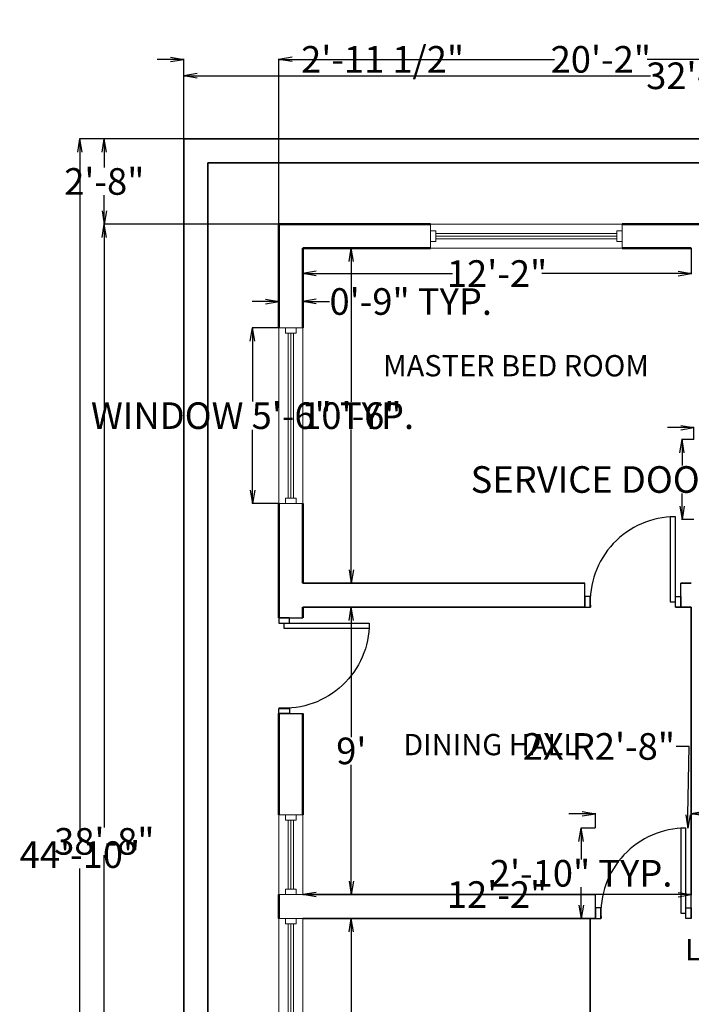
# Model space of a CAD drawing. Units: inches. Extents: x -6539 to -6057, y 19106 to 19733.
# Tile 2 of 3: x -6539 to -6286, y 19363 to 19733. Entities that reach past the tile are written whole.
import ezdxf

# ---------------------------------------------------------------- set-up
doc = ezdxf.new("R2010")
doc.units = ezdxf.units.IN
doc.header["$MEASUREMENT"] = 0
for name, color, linetype, lineweight in [('A-ANNO-DIMS', 121, 'Continuous', 18), ('A-AREA-IDEN', 250, 'Continuous', 25), ('A-WALL-EXTR', 222, 'Continuous', 50), ('C-PROP-WALL', 140, 'Continuous', 35), ('DOORS', 3, 'Continuous', 25), ('interior WALLS', 222, 'Continuous', 35), ('WINDOWS', 20, 'Continuous', 18)]:
    doc.layers.add(name, color=color, linetype=linetype, lineweight=lineweight)
doc.styles.get("Standard").update_dxf_attribs({"font": 'arial.ttf'})
doc.dimstyles.get("Standard").update_dxf_attribs({"dimtxt": 10, "dimasz": 5, "dimexe": 0.18, "dimexo": 0.0625, "dimgap": 0.09, "dimtad": 0, "dimtih": 1, "dimtoh": 1, "dimdec": 0, "dimzin": 0, "dimdsep": 46, "dimlunit": 4, "dimtxsty": 'Standard', "dimblk": 'OPEN', "dimcen": 0.09, "dimadec": 0, "dimazin": 0, "dimtfac": 1, "dimtdec": 0, "dimtofl": 0, "dimtmove": 0, "dimatfit": 0, "dimfxl": 1, "dimtolj": 1, "dimtzin": 0, "dimarcsym": 0})

# ---------------------------------------------------------------- blocks, each defined once
blk = doc.blocks.new('_Open')
at = {"color": 0, "linetype": 'ByBlock', "lineweight": -2}
for p, q in [((-1, 0.167), (0, 0)), ((-1, -0.167), (0, 0)), ((0, 0), (-1, 0))]:
    blk.add_line(p, q, dxfattribs=at)
blk = doc.blocks.new('*D2')
at = {"layer": 'A-ANNO-DIMS', "color": 0, "lineweight": -2, "transparency": 16777216}
for p, q in [((-6476.93, 19688.68), (-6476.93, 19712.48)), ((-6471.93, 19712.3), (-6301.58, 19712.3)), ((-6096.7, 19712.3), (-6267.05, 19712.3)), ((-6091.7, 19688.68), (-6091.7, 19712.48))]:
    blk.add_line(p, q, dxfattribs=at)
at = {"layer": 'Defpoints', "color": 0, "transparency": 16777216}
for p in [(-6091.7, 19712.3), (-6476.93, 19688.62), (-6091.7, 19688.62)]:
    blk.add_point(p, dxfattribs=at)
at = {"layer": 'A-ANNO-DIMS', "color": 0, "lineweight": -2, "transparency": 16777216, "xscale": 5, "yscale": 5, "zscale": 5, "rotation": 180}
blk.add_blockref('_Open', (-6476.93, 19712.3), dxfattribs=at)
at = {"layer": 'A-ANNO-DIMS', "color": 0, "lineweight": -2, "transparency": 16777216, "xscale": 5, "yscale": 5, "zscale": 5}
blk.add_blockref('_Open', (-6091.7, 19712.3), dxfattribs=at)
at = {"layer": 'A-ANNO-DIMS', "color": 0, "transparency": 16777216, "insert": (-6284.31, 19712.3), "char_height": 10, "attachment_point": 5}
blk.add_mtext('\\A1;32\'-1"', dxfattribs=at)
blk = doc.blocks.new('*D3')
at = {"layer": 'A-ANNO-DIMS', "color": 0, "lineweight": -2, "transparency": 16777216}
for p, q in [((-6476.99, 19688.62), (-6516.12, 19688.62)), ((-6515.94, 19683.62), (-6515.94, 19424.78)), ((-6515.94, 19155.56), (-6515.94, 19414.39)), ((-6476.99, 19150.56), (-6516.12, 19150.56))]:
    blk.add_line(p, q, dxfattribs=at)
at = {"layer": 'Defpoints', "color": 0, "transparency": 16777216}
for p in [(-6515.94, 19688.62), (-6476.93, 19688.62), (-6476.93, 19150.56)]:
    blk.add_point(p, dxfattribs=at)
at = {"layer": 'A-ANNO-DIMS', "color": 0, "lineweight": -2, "transparency": 16777216, "xscale": 5, "yscale": 5, "zscale": 5}
for p, rotation in [((-6515.94, 19688.62), 90), ((-6515.94, 19150.56), 270)]:
    blk.add_blockref('_Open', p, dxfattribs=dict(at, rotation=rotation))
at = {"layer": 'A-ANNO-DIMS', "color": 0, "transparency": 16777216, "insert": (-6515.94, 19419.59), "char_height": 10, "attachment_point": 5}
blk.add_mtext('\\A1;44\'-10"', dxfattribs=at)
blk = doc.blocks.new('*D6')
at = {"layer": 'A-ANNO-DIMS', "color": 0, "lineweight": -2, "transparency": 16777216}
for p, q in [((-6432.2, 19647.5), (-6432.2, 19637.79)), ((-6286.2, 19647.5), (-6286.2, 19637.79)), ((-6427.2, 19637.97), (-6376, 19637.97)), ((-6291.2, 19637.97), (-6342.41, 19637.97))]:
    blk.add_line(p, q, dxfattribs=at)
at = {"layer": 'Defpoints', "color": 0, "transparency": 16777216}
for p in [(-6432.2, 19647.56), (-6286.2, 19647.56), (-6286.2, 19637.97)]:
    blk.add_point(p, dxfattribs=at)
at = {"layer": 'A-ANNO-DIMS', "color": 0, "lineweight": -2, "transparency": 16777216, "xscale": 5, "yscale": 5, "zscale": 5, "rotation": 180}
blk.add_blockref('_Open', (-6432.2, 19637.97), dxfattribs=at)
at = {"layer": 'A-ANNO-DIMS', "color": 0, "lineweight": -2, "transparency": 16777216, "xscale": 5, "yscale": 5, "zscale": 5}
blk.add_blockref('_Open', (-6286.2, 19637.97), dxfattribs=at)
at = {"layer": 'A-ANNO-DIMS', "color": 0, "transparency": 16777216, "insert": (-6359.2, 19637.97), "char_height": 10, "attachment_point": 5}
blk.add_mtext('\\A1;12\'-2"', dxfattribs=at)
blk = doc.blocks.new('*D9')
at = {"layer": 'A-ANNO-DIMS', "color": 0, "lineweight": -2, "transparency": 16777216}
for p, q in [((-6432.14, 19647.56), (-6413.78, 19647.56)), ((-6413.96, 19642.56), (-6413.96, 19589.75)), ((-6413.96, 19526.56), (-6413.96, 19579.36)), ((-6432.14, 19521.56), (-6413.78, 19521.56))]:
    blk.add_line(p, q, dxfattribs=at)
at = {"layer": 'Defpoints', "color": 0, "transparency": 16777216}
for p in [(-6432.2, 19647.56), (-6432.2, 19521.56), (-6413.96, 19521.56)]:
    blk.add_point(p, dxfattribs=at)
at = {"layer": 'A-ANNO-DIMS', "color": 0, "lineweight": -2, "transparency": 16777216, "xscale": 5, "yscale": 5, "zscale": 5}
for p, rotation in [((-6413.96, 19647.56), 90), ((-6413.96, 19521.56), 270)]:
    blk.add_blockref('_Open', p, dxfattribs=dict(at, rotation=rotation))
at = {"layer": 'A-ANNO-DIMS', "color": 0, "transparency": 16777216, "insert": (-6413.96, 19584.56), "char_height": 10, "attachment_point": 5}
blk.add_mtext('\\A1;10\'-6"', dxfattribs=at)
blk = doc.blocks.new('*D10')
at = {"layer": 'A-ANNO-DIMS', "color": 0, "lineweight": -2, "transparency": 16777216}
for p, q in [((-6414, 19512.56), (-6414.14, 19512.56)), ((-6413.96, 19507.56), (-6413.96, 19463.75)), ((-6413.96, 19409.56), (-6413.96, 19453.36)), ((-6414.36, 19404.56), (-6413.78, 19404.56))]:
    blk.add_line(p, q, dxfattribs=at)
at = {"layer": 'Defpoints', "color": 0, "transparency": 16777216}
for p in [(-6413.93, 19512.56), (-6414.43, 19404.56), (-6413.96, 19404.56)]:
    blk.add_point(p, dxfattribs=at)
at = {"layer": 'A-ANNO-DIMS', "color": 0, "lineweight": -2, "transparency": 16777216, "xscale": 5, "yscale": 5, "zscale": 5}
for p, rotation in [((-6413.96, 19512.56), 90), ((-6413.96, 19404.56), 270)]:
    blk.add_blockref('_Open', p, dxfattribs=dict(at, rotation=rotation))
at = {"layer": 'A-ANNO-DIMS', "color": 0, "transparency": 16777216, "insert": (-6413.96, 19458.56), "char_height": 10, "attachment_point": 5}
blk.add_mtext("\\A1;9'", dxfattribs=at)
blk = doc.blocks.new('*D11')
at = {"layer": 'A-ANNO-DIMS', "color": 0, "lineweight": -2, "transparency": 16777216}
for p, q in [((-6413.44, 19395.56), (-6414.14, 19395.56)), ((-6413.96, 19390.56), (-6413.96, 19348.75)), ((-6413.96, 19296.56), (-6413.96, 19338.36)), ((-6414.02, 19291.56), (-6413.78, 19291.56))]:
    blk.add_line(p, q, dxfattribs=at)
at = {"layer": 'Defpoints', "color": 0, "transparency": 16777216}
for p in [(-6413.38, 19395.56), (-6414.08, 19291.56), (-6413.96, 19291.56)]:
    blk.add_point(p, dxfattribs=at)
at = {"layer": 'A-ANNO-DIMS', "color": 0, "lineweight": -2, "transparency": 16777216, "xscale": 5, "yscale": 5, "zscale": 5}
for p, rotation in [((-6413.96, 19395.56), 90), ((-6413.96, 19291.56), 270)]:
    blk.add_blockref('_Open', p, dxfattribs=dict(at, rotation=rotation))
at = {"layer": 'A-ANNO-DIMS', "color": 0, "transparency": 16777216, "insert": (-6413.96, 19343.56), "char_height": 10, "attachment_point": 5}
blk.add_mtext('\\A1;8\'-8"', dxfattribs=at)
blk = doc.blocks.new('*D16')
at = {"layer": 'A-ANNO-DIMS', "color": 0, "lineweight": -2, "transparency": 16777216}
for p, q in [((-6432.2, 19404.62), (-6432.2, 19404.74)), ((-6427.2, 19404.56), (-6376, 19404.56)), ((-6291.2, 19404.56), (-6342.41, 19404.56)), ((-6286.2, 19405.11), (-6286.2, 19404.38))]:
    blk.add_line(p, q, dxfattribs=at)
at = {"layer": 'Defpoints', "color": 0, "transparency": 16777216}
for p in [(-6432.2, 19404.56), (-6286.2, 19405.18), (-6286.2, 19404.56)]:
    blk.add_point(p, dxfattribs=at)
at = {"layer": 'A-ANNO-DIMS', "color": 0, "lineweight": -2, "transparency": 16777216, "xscale": 5, "yscale": 5, "zscale": 5, "rotation": 180}
blk.add_blockref('_Open', (-6432.2, 19404.56), dxfattribs=at)
at = {"layer": 'A-ANNO-DIMS', "color": 0, "lineweight": -2, "transparency": 16777216, "xscale": 5, "yscale": 5, "zscale": 5}
blk.add_blockref('_Open', (-6286.2, 19404.56), dxfattribs=at)
at = {"layer": 'A-ANNO-DIMS', "color": 0, "transparency": 16777216, "insert": (-6359.2, 19404.56), "char_height": 10, "attachment_point": 5}
blk.add_mtext('\\A1;12\'-2"', dxfattribs=at)
blk = doc.blocks.new('DOOR-SWING-36IN')
for p, q in [((0, 0), (0, 9)), ((36, 0), (36, 9))]:
    blk.add_line(p, q)
for points in [[(34, 2), (34, 34), (32, 34), (32, 2)], [(0, 0), (2, 0), (2, 4), (0, 4)], [(36, 0), (34, 0), (34, 4), (36, 4)]]:
    blk.add_lwpolyline(points, close=True)
blk.add_arc((34, 2), 32, 90, 183.5833)
blk = doc.blocks.new('WIN-66IN')
for p, q in [((9, 66), (0, 66)), ((0, 66), (0, 0)), ((3.5, 64), (3.5, 2)), ((4.5, 64), (4.5, 2)), ((5.5, 64), (5.5, 2)), ((9, 66), (9, 0)), ((9, 0), (0, 0))]:
    blk.add_line(p, q)
for points in [[(2.5, 66), (2.5, 64), (6.5, 64), (6.5, 66)], [(2.5, 0), (2.5, 2), (6.5, 2), (6.5, 0)]]:
    blk.add_lwpolyline(points, close=True)
blk = doc.blocks.new('*D28')
at = {"layer": 'A-ANNO-DIMS', "color": 0, "lineweight": -2, "transparency": 16777216}
for p, q in [((-6327.2, 19434.96), (-6332.2, 19434.96)), ((-6322.2, 19429.62), (-6322.2, 19435.14)), ((-6286.2, 19429.62), (-6286.2, 19435.14)), ((-6281.2, 19434.96), (-6276.2, 19434.96))]:
    blk.add_line(p, q, dxfattribs=at)
at = {"layer": 'Defpoints', "color": 0, "transparency": 16777216}
for p in [(-6286.2, 19434.96), (-6322.2, 19429.56), (-6286.2, 19429.56)]:
    blk.add_point(p, dxfattribs=at)
at = {"layer": 'A-ANNO-DIMS', "color": 0, "lineweight": -2, "transparency": 16777216, "xscale": 5, "yscale": 5, "zscale": 5}
blk.add_blockref('_Open', (-6322.2, 19434.96), dxfattribs=at)
at = {"layer": 'A-ANNO-DIMS', "color": 0, "lineweight": -2, "transparency": 16777216, "xscale": 5, "yscale": 5, "zscale": 5, "rotation": 180}
blk.add_blockref('_Open', (-6286.2, 19434.96), dxfattribs=at)
at = {"layer": 'A-ANNO-DIMS', "color": 0, "transparency": 16777216, "insert": (-6203.6, 19434.96), "char_height": 10, "attachment_point": 5}
blk.add_mtext('\\A1;HALL DOOR 3\'-0" TYP.', dxfattribs=at)
blk = doc.blocks.new('*D29')
at = {"layer": 'A-ANNO-DIMS', "color": 0, "lineweight": -2, "transparency": 16777216}
for p, q in [((-6322.27, 19429.56), (-6327.78, 19429.56)), ((-6327.6, 19424.56), (-6327.6, 19417.75)), ((-6327.6, 19400.56), (-6327.6, 19407.36)), ((-6322.27, 19395.56), (-6327.78, 19395.56))]:
    blk.add_line(p, q, dxfattribs=at)
at = {"layer": 'Defpoints', "color": 0, "transparency": 16777216}
for p in [(-6327.6, 19429.56), (-6322.2, 19429.56), (-6322.2, 19395.56)]:
    blk.add_point(p, dxfattribs=at)
at = {"layer": 'A-ANNO-DIMS', "color": 0, "lineweight": -2, "transparency": 16777216, "xscale": 5, "yscale": 5, "zscale": 5}
for p, rotation in [((-6327.6, 19429.56), 90), ((-6327.6, 19395.56), 270)]:
    blk.add_blockref('_Open', p, dxfattribs=dict(at, rotation=rotation))
at = {"layer": 'A-ANNO-DIMS', "color": 0, "transparency": 16777216, "insert": (-6327.6, 19412.56), "char_height": 10, "attachment_point": 5}
blk.add_mtext('\\A1;2\'-10" TYP.', dxfattribs=at)
blk = doc.blocks.new('*D30')
at = {"layer": 'A-ANNO-DIMS', "color": 0, "lineweight": -2, "transparency": 16777216}
for p, q in [((-6285.27, 19575.56), (-6289.88, 19575.56)), ((-6289.7, 19570.56), (-6289.7, 19565.82)), ((-6289.7, 19550.56), (-6289.7, 19555.29)), ((-6285.27, 19545.56), (-6289.88, 19545.56))]:
    blk.add_line(p, q, dxfattribs=at)
at = {"layer": 'Defpoints', "color": 0, "transparency": 16777216}
for p in [(-6289.7, 19575.56), (-6285.2, 19575.56), (-6285.2, 19545.56)]:
    blk.add_point(p, dxfattribs=at)
at = {"layer": 'A-ANNO-DIMS', "color": 0, "lineweight": -2, "transparency": 16777216, "xscale": 5, "yscale": 5, "zscale": 5}
for p, rotation in [((-6289.7, 19575.56), 90), ((-6289.7, 19545.56), 270)]:
    blk.add_blockref('_Open', p, dxfattribs=dict(at, rotation=rotation))
at = {"layer": 'A-ANNO-DIMS', "color": 0, "transparency": 16777216, "insert": (-6289.7, 19560.56), "char_height": 10, "attachment_point": 5}
blk.add_mtext('\\A1;SERVICE DOOR 2\'-6" TYP.', dxfattribs=at)
blk = doc.blocks.new('*D31')
at = {"layer": 'A-ANNO-DIMS', "color": 0, "lineweight": -2, "transparency": 16777216}
for p, q in [((-6290.2, 19580.06), (-6295.2, 19580.06)), ((-6285.2, 19575.62), (-6285.2, 19580.24)), ((-6257.2, 19575.62), (-6257.2, 19580.24)), ((-6252.2, 19580.06), (-6247.2, 19580.06))]:
    blk.add_line(p, q, dxfattribs=at)
at = {"layer": 'Defpoints', "color": 0, "transparency": 16777216}
for p in [(-6257.2, 19580.06), (-6285.2, 19575.56), (-6257.2, 19575.56)]:
    blk.add_point(p, dxfattribs=at)
at = {"layer": 'A-ANNO-DIMS', "color": 0, "lineweight": -2, "transparency": 16777216, "xscale": 5, "yscale": 5, "zscale": 5}
blk.add_blockref('_Open', (-6285.2, 19580.06), dxfattribs=at)
at = {"layer": 'A-ANNO-DIMS', "color": 0, "lineweight": -2, "transparency": 16777216, "xscale": 5, "yscale": 5, "zscale": 5, "rotation": 180}
blk.add_blockref('_Open', (-6257.2, 19580.06), dxfattribs=at)
at = {"layer": 'A-ANNO-DIMS', "color": 0, "transparency": 16777216, "insert": (-6216.55, 19580.06), "char_height": 10, "attachment_point": 5}
blk.add_mtext('\\A1;2\'-4" TYP.', dxfattribs=at)
blk = doc.blocks.new('*D34')
at = {"layer": 'A-ANNO-DIMS', "color": 0, "lineweight": -2, "transparency": 16777216}
for p, q in [((-6441.27, 19617.56), (-6451.28, 19617.56)), ((-6451.1, 19612.56), (-6451.1, 19589.82)), ((-6451.1, 19556.56), (-6451.1, 19579.29)), ((-6441.27, 19551.56), (-6451.28, 19551.56))]:
    blk.add_line(p, q, dxfattribs=at)
at = {"layer": 'Defpoints', "color": 0, "transparency": 16777216}
for p in [(-6451.1, 19617.56), (-6441.2, 19617.56), (-6441.2, 19551.56)]:
    blk.add_point(p, dxfattribs=at)
at = {"layer": 'A-ANNO-DIMS', "color": 0, "lineweight": -2, "transparency": 16777216, "xscale": 5, "yscale": 5, "zscale": 5}
for p, rotation in [((-6451.1, 19617.56), 90), ((-6451.1, 19551.56), 270)]:
    blk.add_blockref('_Open', p, dxfattribs=dict(at, rotation=rotation))
at = {"layer": 'A-ANNO-DIMS', "color": 0, "transparency": 16777216, "insert": (-6451.1, 19584.56), "char_height": 10, "attachment_point": 5}
blk.add_mtext('\\A1;WINDOW 5\'-6" TYP.', dxfattribs=at)
blk = doc.blocks.new('*D35')
at = {"layer": 'A-ANNO-DIMS', "color": 0, "lineweight": -2, "transparency": 16777216}
for p, q in [((-6446.2, 19627.46), (-6451.2, 19627.46)), ((-6441.2, 19617.62), (-6441.2, 19627.64)), ((-6432.2, 19617.62), (-6432.2, 19627.64)), ((-6427.2, 19627.46), (-6422.2, 19627.46))]:
    blk.add_line(p, q, dxfattribs=at)
at = {"layer": 'Defpoints', "color": 0, "transparency": 16777216}
for p in [(-6432.2, 19627.46), (-6441.2, 19617.56), (-6432.2, 19617.56)]:
    blk.add_point(p, dxfattribs=at)
at = {"layer": 'A-ANNO-DIMS', "color": 0, "lineweight": -2, "transparency": 16777216, "xscale": 5, "yscale": 5, "zscale": 5}
blk.add_blockref('_Open', (-6441.2, 19627.46), dxfattribs=at)
at = {"layer": 'A-ANNO-DIMS', "color": 0, "lineweight": -2, "transparency": 16777216, "xscale": 5, "yscale": 5, "zscale": 5, "rotation": 180}
blk.add_blockref('_Open', (-6432.2, 19627.46), dxfattribs=at)
at = {"layer": 'A-ANNO-DIMS', "color": 0, "transparency": 16777216, "insert": (-6391.64, 19627.46), "char_height": 10, "attachment_point": 5}
blk.add_mtext('\\A1;0\'-9" TYP.', dxfattribs=at)
blk = doc.blocks.new('*D36')
at = {"layer": 'A-ANNO-DIMS', "color": 0, "lineweight": -2, "transparency": 16777216}
for p, q in [((-6481.93, 19718.47), (-6486.93, 19718.47)), ((-6476.93, 19688.68), (-6476.93, 19718.65)), ((-6441.2, 19656.62), (-6441.2, 19718.65)), ((-6436.2, 19718.47), (-6431.2, 19718.47))]:
    blk.add_line(p, q, dxfattribs=at)
at = {"layer": 'Defpoints', "color": 0, "transparency": 16777216}
for p in [(-6441.2, 19718.47), (-6476.93, 19688.62), (-6441.2, 19656.56)]:
    blk.add_point(p, dxfattribs=at)
at = {"layer": 'A-ANNO-DIMS', "color": 0, "lineweight": -2, "transparency": 16777216, "xscale": 5, "yscale": 5, "zscale": 5}
blk.add_blockref('_Open', (-6476.93, 19718.47), dxfattribs=at)
at = {"layer": 'A-ANNO-DIMS', "color": 0, "lineweight": -2, "transparency": 16777216, "xscale": 5, "yscale": 5, "zscale": 5, "rotation": 180}
blk.add_blockref('_Open', (-6441.2, 19718.47), dxfattribs=at)
at = {"layer": 'A-ANNO-DIMS', "color": 0, "transparency": 16777216, "insert": (-6402.2, 19718.47), "char_height": 10, "attachment_point": 5}
blk.add_mtext('\\A1;2\'-11 1/2"', dxfattribs=at)
blk = doc.blocks.new('*D37')
at = {"layer": 'A-ANNO-DIMS', "color": 0, "lineweight": -2, "transparency": 16777216}
for p, q in [((-6476.99, 19688.62), (-6506.96, 19688.62)), ((-6506.78, 19683.62), (-6506.78, 19677.78)), ((-6506.78, 19661.56), (-6506.78, 19667.39)), ((-6441.27, 19656.56), (-6506.96, 19656.56))]:
    blk.add_line(p, q, dxfattribs=at)
at = {"layer": 'Defpoints', "color": 0, "transparency": 16777216}
for p in [(-6476.93, 19688.62), (-6506.78, 19656.56), (-6441.2, 19656.56)]:
    blk.add_point(p, dxfattribs=at)
at = {"layer": 'A-ANNO-DIMS', "color": 0, "lineweight": -2, "transparency": 16777216, "xscale": 5, "yscale": 5, "zscale": 5}
for p, rotation in [((-6506.78, 19688.62), 90), ((-6506.78, 19656.56), 270)]:
    blk.add_blockref('_Open', p, dxfattribs=dict(at, rotation=rotation))
at = {"layer": 'A-ANNO-DIMS', "color": 0, "transparency": 16777216, "insert": (-6506.78, 19672.59), "char_height": 10, "attachment_point": 5}
blk.add_mtext('\\A1;2\'-8"', dxfattribs=at)
blk = doc.blocks.new('*D38')
at = {"layer": 'A-ANNO-DIMS', "color": 0, "lineweight": -2, "transparency": 16777216}
for p, q in [((-6441.2, 19656.62), (-6441.2, 19718.65)), ((-6436.2, 19718.47), (-6337.56, 19718.47)), ((-6204.2, 19718.47), (-6302.85, 19718.47)), ((-6199.2, 19656.62), (-6199.2, 19718.65))]:
    blk.add_line(p, q, dxfattribs=at)
at = {"layer": 'Defpoints', "color": 0, "transparency": 16777216}
for p in [(-6199.2, 19718.47), (-6441.2, 19656.56), (-6199.2, 19656.56)]:
    blk.add_point(p, dxfattribs=at)
at = {"layer": 'A-ANNO-DIMS', "color": 0, "lineweight": -2, "transparency": 16777216, "xscale": 5, "yscale": 5, "zscale": 5, "rotation": 180}
blk.add_blockref('_Open', (-6441.2, 19718.47), dxfattribs=at)
at = {"layer": 'A-ANNO-DIMS', "color": 0, "lineweight": -2, "transparency": 16777216, "xscale": 5, "yscale": 5, "zscale": 5}
blk.add_blockref('_Open', (-6199.2, 19718.47), dxfattribs=at)
at = {"layer": 'A-ANNO-DIMS', "color": 0, "transparency": 16777216, "insert": (-6320.2, 19718.47), "char_height": 10, "attachment_point": 5}
blk.add_mtext('\\A1;20\'-2"', dxfattribs=at)
blk = doc.blocks.new('*D39')
at = {"layer": 'A-ANNO-DIMS', "color": 0, "lineweight": -2, "transparency": 16777216}
for p, q in [((-6441.27, 19656.56), (-6506.96, 19656.56)), ((-6506.78, 19651.56), (-6506.78, 19429.76)), ((-6506.78, 19197.56), (-6506.78, 19419.36)), ((-6441.27, 19192.56), (-6506.96, 19192.56))]:
    blk.add_line(p, q, dxfattribs=at)
at = {"layer": 'Defpoints', "color": 0, "transparency": 16777216}
for p in [(-6441.2, 19656.56), (-6506.78, 19192.56), (-6441.2, 19192.56)]:
    blk.add_point(p, dxfattribs=at)
at = {"layer": 'A-ANNO-DIMS', "color": 0, "lineweight": -2, "transparency": 16777216, "xscale": 5, "yscale": 5, "zscale": 5}
for p, rotation in [((-6506.78, 19656.56), 90), ((-6506.78, 19192.56), 270)]:
    blk.add_blockref('_Open', p, dxfattribs=dict(at, rotation=rotation))
at = {"layer": 'A-ANNO-DIMS', "color": 0, "transparency": 16777216, "insert": (-6506.78, 19424.56), "char_height": 10, "attachment_point": 5}
blk.add_mtext('\\A1;38\'-8"', dxfattribs=at)
blk = doc.blocks.new('*D42')
at = {"layer": 'A-ANNO-DIMS', "color": 0, "lineweight": -2, "transparency": 16777216}
for p, q in [((-6286.95, 19460.24), (-6291.95, 19460.24)), ((-6287.46, 19434.55), (-6286.95, 19460.24)), ((-6288.29, 19397.56), (-6288.11, 19397.56)), ((-6288.2, 19397.47), (-6288.2, 19397.65))]:
    blk.add_line(p, q, dxfattribs=at)
at = {"layer": 'Defpoints', "color": 0, "transparency": 16777216}
for p in [(-6287.56, 19429.55), (-6288.2, 19397.56)]:
    blk.add_point(p, dxfattribs=at)
at = {"layer": 'A-ANNO-DIMS', "color": 0, "lineweight": -2, "transparency": 16777216, "xscale": 5, "yscale": 5, "zscale": 5, "rotation": 268.8501996189172}
blk.add_blockref('_Open', (-6287.56, 19429.55), dxfattribs=at)
at = {"layer": 'A-ANNO-DIMS', "color": 0, "transparency": 16777216, "insert": (-6320.94, 19460.24), "char_height": 10, "attachment_point": 5}
blk.add_mtext('\\A1;2X R2\'-8"', dxfattribs=at)

msp = doc.modelspace()

# ---------------------------------------------------------------- linework, layer by layer
at = {"layer": 'A-WALL-EXTR'}
for p, q in [((-6441.2, 19656.56), (-6441.2, 19617.56)), ((-6441.2, 19656.56), (-6384.2, 19656.56)), ((-6312.2, 19656.56), (-6255.2, 19656.56)), ((-6432.2, 19647.56), (-6384.2, 19647.56)), ((-6432.2, 19617.56), (-6432.2, 19647.56)), ((-6312.2, 19647.56), (-6286.2, 19647.56)), ((-6441.2, 19508.56), (-6441.2, 19551.56)), ((-6441.2, 19551.56), (-6441.2, 19508.56)), ((-6432.2, 19521.56), (-6432.2, 19551.56)), ((-6432.2, 19508.56), (-6432.2, 19512.56)), ((-6441.2, 19472.56), (-6441.2, 19434.56)), ((-6441.2, 19434.56), (-6441.2, 19472.56)), ((-6432.2, 19434.56), (-6432.2, 19472.56)), ((-6441.2, 19395.56), (-6441.2, 19404.56)), ((-6441.2, 19404.56), (-6441.2, 19395.56))]:
    msp.add_line(p, q, dxfattribs=at)
at = {"layer": 'C-PROP-WALL'}
for p, q in [((-6476.93, 19688.62), (-6476.93, 19483.62)), ((-6476.93, 19688.62), (-6476.93, 19150.56)), ((-6476.93, 19688.62), (-6091.7, 19688.62)), ((-6467.93, 19679.62), (-6467.93, 19159.56)), ((-6467.93, 19679.62), (-6205.2, 19679.62))]:
    msp.add_line(p, q, dxfattribs=at)
at = {"layer": 'DOORS'}
for p, q in [((-6326.2, 19512.56), (-6324.14, 19512.56)), ((-6292.2, 19512.56), (-6290.2, 19512.56))]:
    msp.add_line(p, q, dxfattribs=at)
at = {"layer": 'interior WALLS'}
for p, q in [((-6432.2, 19521.56), (-6326.2, 19521.56)), ((-6290.2, 19521.56), (-6286.2, 19521.56)), ((-6432.2, 19512.56), (-6326.2, 19512.56)), ((-6290.2, 19512.56), (-6286.2, 19512.56)), ((-6286.2, 19404.56), (-6286.2, 19512.56)), ((-6432.2, 19404.56), (-6322.2, 19404.56)), ((-6432.2, 19395.56), (-6322.2, 19395.56)), ((-6324.2, 19337.56), (-6324.2, 19395.56))]:
    msp.add_line(p, q, dxfattribs=at)
at = {"layer": 'WINDOWS'}
for p, q in [((-6384.2, 19647.56), (-6384.2, 19656.56)), ((-6384.2, 19656.56), (-6312.2, 19656.56)), ((-6312.2, 19647.56), (-6312.2, 19656.56)), ((-6382.2, 19653.06), (-6314.2, 19653.06)), ((-6382.2, 19652.06), (-6314.2, 19652.06)), ((-6382.2, 19651.06), (-6314.2, 19651.06)), ((-6384.2, 19647.56), (-6312.2, 19647.56)), ((-6441.2, 19434.7), (-6441.2, 19404.56)), ((-6432.2, 19434.56), (-6441.2, 19434.56)), ((-6437.7, 19432.56), (-6437.7, 19406.56)), ((-6436.7, 19432.56), (-6436.7, 19406.56)), ((-6435.7, 19432.56), (-6435.7, 19406.56)), ((-6432.2, 19434.7), (-6432.2, 19404.56)), ((-6432.2, 19404.56), (-6441.2, 19404.56))]:
    msp.add_line(p, q, dxfattribs=at)
for points in [[(-6384.2, 19650.06), (-6382.2, 19650.06), (-6382.2, 19654.06), (-6384.2, 19654.06)], [(-6312.2, 19650.06), (-6314.2, 19650.06), (-6314.2, 19654.06), (-6312.2, 19654.06)], [(-6438.7, 19432.56), (-6434.7, 19432.56), (-6434.7, 19434.56), (-6438.7, 19434.56)], [(-6438.7, 19406.56), (-6434.7, 19406.56), (-6434.7, 19404.56), (-6438.7, 19404.56)]]:
    msp.add_lwpolyline(points, close=True, dxfattribs=at)

# ---------------------------------------------------------------- block references
at = {"layer": 'DOORS'}
for p in [(-6326.2, 19512.56), (-6322.2, 19395.56)]:
    msp.add_blockref('DOOR-SWING-36IN', p, dxfattribs=at)
at = {"layer": 'DOORS', "extrusion": (0, 0, -1), "zscale": -1, "rotation": 89.99999999999199}
msp.add_blockref('DOOR-SWING-36IN', (6441.2, 19472.56), dxfattribs=at)
at = {"layer": 'WINDOWS'}
for p in [(-6441.2, 19551.56), (-6441.2, 19329.56)]:
    msp.add_blockref('WIN-66IN', p, dxfattribs=at)

# ---------------------------------------------------------------- texts
at = {"layer": 'A-AREA-IDEN'}
for s, p in [('MASTER BED ROOM ', (-6402.03, 19599.33)), (' DINING HALL', (-6396.9, 19456.93)), ('LIVING HALL ', (-6288.56, 19379.83))]:
    msp.add_text(s, height=8, dxfattribs=at).set_placement(p)

# ---------------------------------------------------------------- dimensions: what is measured, and where the dimension line sits
at = {"layer": 'A-ANNO-DIMS'}
for base, p1, p2, override, picture, middle in [((-6441.2, 19718.47), (-6476.93, 19688.62), (-6441.2, 19656.56), {"dimdec": 1, "dimlfac": 1, "dimrnd": 0, "dimzin": 1, "dimdsep": 46, "dimlunit": 4, "dimfrac": 2}, '*D36', (-6402.2, 19718.47)), ((-6199.2, 19718.47), (-6441.2, 19656.56), (-6199.2, 19656.56), {"dimdec": 1, "dimlfac": 1, "dimrnd": 0, "dimzin": 1, "dimdsep": 46, "dimlunit": 4, "dimfrac": 2}, '*D38', (-6320.2, 19718.47)), ((-6091.7, 19712.3), (-6476.93, 19688.62), (-6091.7, 19688.62), {"dimclrd": 0, "dimclre": 0, "dimclrt": 0}, '*D2', (-6284.31, 19712.3)), ((-6286.2, 19637.97), (-6432.2, 19647.56), (-6286.2, 19647.56), {"dimclrd": 0, "dimclre": 0, "dimclrt": 0}, '*D6', (-6359.2, 19637.97)), ((-6286.2, 19404.56), (-6432.2, 19404.56), (-6286.2, 19405.18), {"dimclrd": 0, "dimclre": 0, "dimclrt": 0}, '*D16', (-6359.2, 19404.56))]:
    dim = msp.add_linear_dim(base=base, p1=p1, p2=p2, dimstyle='Standard', override=override, dxfattribs=at)
    dim.commit()
    dim.dimension.update_dxf_attribs({"geometry": picture, "text_midpoint": middle})
for base, p1, p2, override, picture, middle in [((-6515.94, 19688.62), (-6476.93, 19150.56), (-6476.93, 19688.62), {"dimclrd": 0, "dimclre": 0, "dimclrt": 0}, '*D3', (-6515.94, 19419.59)), ((-6506.78, 19656.56), (-6476.93, 19688.62), (-6441.2, 19656.56), {"dimdec": 1, "dimlfac": 1, "dimrnd": 0, "dimzin": 1, "dimdsep": 46, "dimlunit": 4, "dimfrac": 2}, '*D37', (-6506.78, 19672.59)), ((-6506.78, 19192.56), (-6441.2, 19656.56), (-6441.2, 19192.56), {"dimdec": 1, "dimlfac": 1, "dimrnd": 0, "dimzin": 1, "dimdsep": 46, "dimlunit": 4, "dimfrac": 2}, '*D39', (-6506.78, 19424.56)), ((-6413.96, 19521.56), (-6432.2, 19647.56), (-6432.2, 19521.56), {"dimclrd": 0, "dimclre": 0, "dimclrt": 0}, '*D9', (-6413.96, 19584.56)), ((-6413.96, 19404.56), (-6413.93, 19512.56), (-6414.43, 19404.56), {"dimclrd": 0, "dimclre": 0, "dimclrt": 0, "dimtmove": 1}, '*D10', (-6413.96, 19458.56)), ((-6413.96, 19291.56), (-6413.38, 19395.56), (-6414.08, 19291.56), {"dimclrd": 0, "dimclre": 0, "dimclrt": 0, "dimtmove": 1}, '*D11', (-6413.96, 19343.56))]:
    dim = msp.add_linear_dim(base=base, p1=p1, p2=p2, angle=90, dimstyle='Standard', override=override, dxfattribs=at)
    dim.commit()
    dim.dimension.update_dxf_attribs({"geometry": picture, "text_midpoint": middle})
for base, p1, p2, text, picture, middle in [((-6432.2, 19627.46), (-6441.2, 19617.56), (-6432.2, 19617.56), '<> TYP.', '*D35', (-6391.64, 19627.46)), ((-6257.2, 19580.06), (-6285.2, 19575.56), (-6257.2, 19575.56), '<> TYP.', '*D31', (-6216.55, 19580.06)), ((-6286.2, 19434.96), (-6322.2, 19429.56), (-6286.2, 19429.56), 'HALL DOOR <> TYP.', '*D28', (-6203.6, 19434.96))]:
    dim = msp.add_linear_dim(base=base, p1=p1, p2=p2, text=text, dimstyle='Standard', override={"dimdec": 1, "dimlfac": 1, "dimrnd": 0, "dimzin": 1, "dimdsep": 46, "dimlunit": 4, "dimfrac": 2}, dxfattribs=at)
    dim.commit()
    dim.dimension.update_dxf_attribs({"geometry": picture, "text_midpoint": middle})
for base, p1, p2, text, picture, middle in [((-6451.1, 19617.56), (-6441.2, 19551.56), (-6441.2, 19617.56), 'WINDOW <> TYP.', '*D34', (-6451.1, 19584.56)), ((-6289.7, 19575.56), (-6285.2, 19545.56), (-6285.2, 19575.56), 'SERVICE DOOR <> TYP.', '*D30', (-6289.7, 19560.56)), ((-6327.6, 19429.56), (-6322.2, 19395.56), (-6322.2, 19429.56), '<> TYP.', '*D29', (-6327.6, 19412.56))]:
    dim = msp.add_linear_dim(base=base, p1=p1, p2=p2, angle=90, text=text, dimstyle='Standard', override={"dimdec": 1, "dimlfac": 1, "dimrnd": 0, "dimzin": 1, "dimdsep": 46, "dimlunit": 4, "dimfrac": 2}, dxfattribs=at)
    dim.commit()
    dim.dimension.update_dxf_attribs({"geometry": picture, "text_midpoint": middle})
dim = msp.add_radius_dim(center=(-6288.2, 19397.56), mpoint=(-6287.56, 19429.55), text='2X <>', dimstyle='Standard', override={"dimdec": 1, "dimlfac": 1, "dimrnd": 0, "dimzin": 1, "dimdsep": 46, "dimlunit": 4, "dimfrac": 2}, dxfattribs=at)
dim.commit()
dim.dimension.update_dxf_attribs({"geometry": '*D42', "text_midpoint": (-6320.94, 19460.24), "dimtype": 164})

doc.saveas('drawing.dxf')
